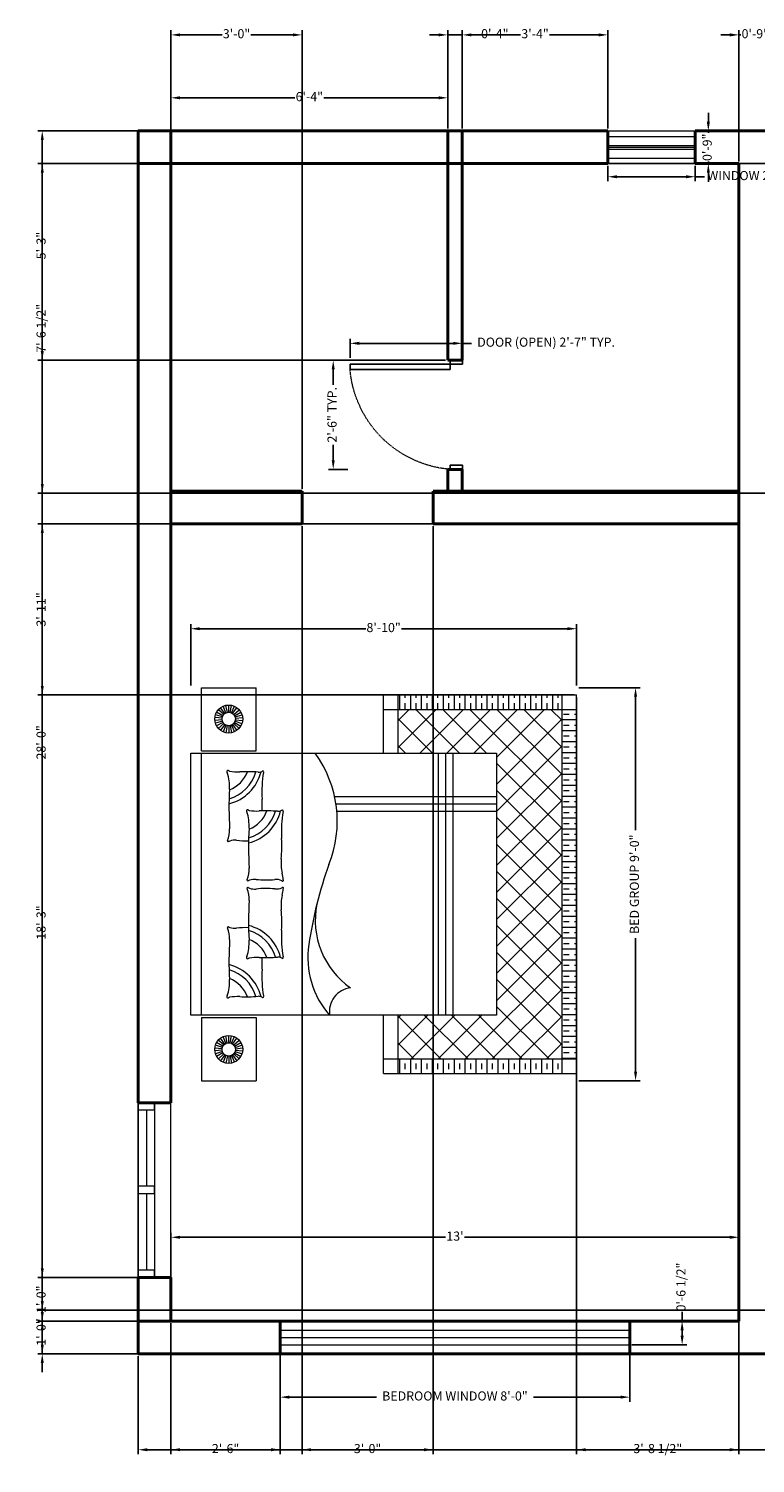
# Model space of a CAD drawing. Units: inches. Extents: x 3502 to 4078, y 3147 to 3541.
# Tile 1 of 3: x 3502 to 3702, y 3147 to 3541. Entities that reach past the tile are written whole.
import ezdxf

# ---------------------------------------------------------------- set-up
doc = ezdxf.new("R2010")
doc.units = ezdxf.units.IN
doc.linetypes.add('HIDDEN4', pattern=[0.09375, 0.0625, -0.03125])
doc.layers.get('0').update_dxf_attribs({"color": 255})
for name, color, linetype, lineweight in [('A-ANNO-DIMS', 2, 'Continuous', 18), ('A-FURN', 8, 'Continuous', 18), ('A-WALL', 7, 'Continuous', 40), ('A-WINDOW', 5, 'Continuous', 15)]:
    doc.layers.add(name, color=color, linetype=linetype, lineweight=lineweight)
doc.layers.add('A-DOOR', color=32, linetype='Continuous', lineweight=25, true_color=0xcd6928)
doc.layers.add('A-DOOR-SWNG', color=32, linetype='HIDDEN4', lineweight=13, true_color=0xcd6928)
doc.styles.get("Standard").update_dxf_attribs({"font": 'arial.ttf'})
doc.dimstyles.new('ISO-25', dxfattribs={"dimtxt": 2.5, "dimasz": 2.5, "dimexe": 1.25, "dimexo": 0.625, "dimtad": 0, "dimlunit": 4, "dimtxsty": 'Standard', "dimcen": 2.5, "dimadec": 0, "dimazin": 0, "dimtfac": 1, "dimtmove": 0, "dimatfit": 3, "dimfxl": 1, "dimarcsym": 0})

# ---------------------------------------------------------------- blocks, each defined once
blk = doc.blocks.new('*D2')
at = {"layer": 'A-ANNO-DIMS', "color": 0, "lineweight": -2, "transparency": 16777216}
for p, q in [((3541.21, 3513.35), (3541.21, 3523.06)), ((3543.71, 3521.81), (3575.25, 3521.81)), ((3614.71, 3521.81), (3583.16, 3521.81)), ((3617.21, 3513.35), (3617.21, 3523.06))]:
    blk.add_line(p, q, dxfattribs=at)
at = {"layer": 'A-ANNO-DIMS', "color": 0, "transparency": 16777216}
for points in [[(3543.71, 3522.23), (3543.71, 3521.39), (3541.21, 3521.81)], [(3614.71, 3522.23), (3614.71, 3521.39), (3617.21, 3521.81)]]:
    blk.add_solid(points, dxfattribs=at)
at = {"layer": 'Defpoints', "color": 0, "transparency": 16777216}
for p in [(3617.21, 3521.81), (3541.21, 3512.72), (3617.21, 3512.72)]:
    blk.add_point(p, dxfattribs=at)
at = {"layer": 'A-ANNO-DIMS', "color": 0, "transparency": 16777216, "insert": (3579.21, 3521.81), "char_height": 2.5, "attachment_point": 5}
blk.add_mtext('6\'-4"', dxfattribs=at)
blk = doc.blocks.new('A$C63CB6BFC')
at = {"layer": 'A-WALL', "ltscale": 75}
for p, q in [((0, 9), (0, 0)), ((48, 9), (48, 0))]:
    blk.add_line(p, q, dxfattribs=at)
at = {"layer": 'A-WINDOW'}
for p, q in [((48, 9), (0, 9)), ((0, 9), (48, 9)), ((1.99, 4.5), (1.99, 9)), ((23.04, 9), (23.04, 4.5)), ((25.02, 4.5), (25.02, 9)), ((46.01, 9), (46.01, 4.5)), ((48, 4.5), (0, 4.5)), ((0, 4.5), (1.99, 4.5)), ((23.04, 6.75), (1.99, 6.75)), ((23.04, 4.5), (25.02, 4.5)), ((46.01, 6.75), (25.02, 6.75)), ((46.01, 4.5), (48, 4.5)), ((0, 0), (48, 0))]:
    blk.add_line(p, q, dxfattribs=at)
blk = doc.blocks.new('*D9')
at = {"layer": 'A-ANNO-DIMS', "color": 0, "lineweight": -2, "transparency": 16777216}
for p, q in [((3541.21, 3186.35), (3541.21, 3209.99)), ((3543.71, 3208.74), (3616.58, 3208.74)), ((3694.71, 3208.74), (3621.84, 3208.74)), ((3697.21, 3186.35), (3697.21, 3209.99))]:
    blk.add_line(p, q, dxfattribs=at)
at = {"layer": 'A-ANNO-DIMS', "color": 0, "transparency": 16777216}
for points in [[(3543.71, 3209.16), (3543.71, 3208.33), (3541.21, 3208.74)], [(3694.71, 3209.16), (3694.71, 3208.33), (3697.21, 3208.74)]]:
    blk.add_solid(points, dxfattribs=at)
at = {"layer": 'Defpoints', "color": 0, "transparency": 16777216}
for p in [(3697.21, 3208.74), (3541.21, 3185.72), (3697.21, 3185.72)]:
    blk.add_point(p, dxfattribs=at)
at = {"layer": 'A-ANNO-DIMS', "color": 0, "transparency": 16777216, "insert": (3619.21, 3208.74), "char_height": 2.5, "attachment_point": 5}
blk.add_mtext("13'", dxfattribs=at)
blk = doc.blocks.new('BED')
h = blk.add_hatch()
h.set_pattern_fill('TRANS', color=256, scale=12, style=0)
h.set_pattern_definition([(360, (4433.967, -9715.0492), (1e-15, 3), []), (360, (4433.967, -9713.5492), (1e-15, 3), [1.5, -1.5])])
h.paths.add_polyline_path([(48, -103), (52, -103), (52, -58), (48, -58)])
h.paths.add_polyline_path([(-48, -58), (-52, -58), (-52, -103), (-48, -103)])
h = blk.add_hatch()
h.set_pattern_fill('ANSI37', color=256, scale=42, angle=-90, style=0)
h.set_pattern_definition([(315, (7787.1367, 4477.8466), (3.7123106, 3.7123106), []), (45, (7787.1367, 4477.8466), (-3.7123106, 3.7123106), [])])
h.paths.add_polyline_path([(-36, -85), (-36, -58), (-48, -58), (-48, -103), (48, -103), (48, -58), (36, -58), (36, -85)])
h = blk.add_hatch()
h.set_pattern_fill('TRANS', color=256, scale=12, angle=-90, style=0)
h.set_pattern_definition([(270, (4433.967, -9715.0492), (3, -1e-15), []), (270, (4435.467, -9715.0492), (3, -1e-15), [1.5, -1.5])])
h.paths.add_polyline_path([(48, -107), (48, -103), (-48, -103), (-48, -107)])
for p, q in [((-36, -1), (36, -1)), ((-36, -85), (-36, -1)), ((36, -1), (36, -85)), ((-54, -4), (-54, -19)), ((-36.64, -4), (-54, -4)), ((-45.96, -9.7), (-46.58, -7.8)), ((-45.58, -9.62), (-45.8, -7.63)), ((-45.2, -9.62), (-45, -7.63)), ((-44.82, -9.7), (-44.21, -7.79)), ((-36.64, -4), (-36.64, -19)), ((-36, -4), (36, -4)), ((36.64, -4), (36.64, -19)), ((36.64, -4), (54, -4)), ((44.82, -9.7), (44.21, -7.79)), ((45.2, -9.62), (45, -7.63)), ((45.58, -9.62), (45.8, -7.63)), ((45.96, -9.7), (46.58, -7.8)), ((54, -4), (54, -19)), ((-47.23, -11.45), (-49.23, -11.45)), ((-47.19, -11.07), (-49.14, -10.66)), ((-47.07, -10.7), (-48.9, -9.89)), ((-46.88, -10.37), (-48.5, -9.2)), ((-46.62, -10.08), (-47.96, -8.6)), ((-46.31, -9.86), (-47.31, -8.13)), ((-44.47, -9.85), (-43.48, -8.12)), ((-44.16, -10.08), (-42.83, -8.59)), ((-43.9, -10.36), (-42.29, -9.18)), ((-43.71, -10.7), (-41.89, -9.88)), ((-43.59, -11.06), (-41.64, -10.64)), ((-43.55, -11.44), (-41.55, -11.44)), ((43.55, -11.44), (41.55, -11.44)), ((43.59, -11.06), (41.64, -10.64)), ((43.71, -10.7), (41.89, -9.88)), ((43.9, -10.36), (42.29, -9.18)), ((44.16, -10.08), (42.83, -8.59)), ((44.47, -9.85), (43.48, -8.12)), ((46.31, -9.86), (47.31, -8.13)), ((46.62, -10.08), (47.96, -8.6)), ((46.88, -10.37), (48.5, -9.2)), ((47.07, -10.7), (48.9, -9.89)), ((47.19, -11.07), (49.14, -10.66)), ((47.23, -11.45), (49.23, -11.45)), ((-47.19, -11.83), (-49.14, -12.25)), ((-47.07, -12.2), (-48.89, -13.01)), ((-46.87, -12.53), (-48.49, -13.71)), ((-46.62, -12.81), (-47.95, -14.3)), ((-46.3, -13.04), (-47.3, -14.77)), ((-45.95, -13.2), (-46.57, -15.1)), ((-45.58, -13.27), (-45.78, -15.26)), ((-45.19, -13.27), (-44.98, -15.26)), ((-44.82, -13.19), (-44.2, -15.09)), ((-44.47, -13.04), (-43.46, -14.77)), ((-44.16, -12.81), (-42.82, -14.29)), ((-43.9, -12.52), (-42.28, -13.7)), ((-43.71, -12.19), (-41.88, -13)), ((-43.59, -11.83), (-41.63, -12.24)), ((43.59, -11.83), (41.63, -12.24)), ((43.71, -12.19), (41.88, -13)), ((43.9, -12.52), (42.28, -13.7)), ((44.16, -12.81), (42.82, -14.29)), ((44.47, -13.04), (43.46, -14.77)), ((44.82, -13.19), (44.2, -15.09)), ((45.19, -13.27), (44.98, -15.26)), ((45.58, -13.27), (45.78, -15.26)), ((45.95, -13.2), (46.57, -15.1)), ((46.3, -13.04), (47.3, -14.77)), ((46.62, -12.81), (47.95, -14.3)), ((46.87, -12.53), (48.49, -13.71)), ((47.07, -12.2), (48.89, -13.01)), ((47.19, -11.83), (49.14, -12.25)), ((-36.64, -19), (-54, -19)), ((36.64, -19), (54, -19)), ((20, -85), (20, -41.14)), ((22, -85), (22, -40.91)), ((24, -85), (24, -40.55)), ((-52, -54), (-52, -107)), ((-52, -54), (-36, -54)), ((-48, -54), (-48, -107)), ((36, -54), (52, -54)), ((48, -54), (48, -107)), ((52, -54), (52, -107)), ((-52, -58), (-36, -58)), ((36, -58), (52, -58)), ((36, -69), (-36, -69)), ((36, -71), (-36, -71)), ((36, -73), (-36, -73)), ((36, -85), (-36, -85)), ((-52, -103), (52, -103)), ((-52, -107), (52, -107))]:
    blk.add_line(p, q)
for centre, radius in [((-45.39, -11.45), 3.84), ((45.39, -11.45), 3.84), ((-45.39, -11.45), 1.84), ((45.39, -11.45), 1.84)]:
    blk.add_circle(centre, radius)
for centre, radius, start, end in [((-30.92, -11.24), 0.328, 35.8976, 208.6272), ((-42.38, -17.5), 12.73, 27.1629, 28.6272), ((-44.37, -13.89), 13.5, 357.4804, 9.3956), ((-33.8, -8.61), 8.46, 289.8695, 338.9843), ((-33.8, -8.61), 12.06, 283.8498, 346.0842), ((-33.8, -8.61), 10.71, 286.0319, 344.1205), ((-26.84, 0.13), 11.82, 251.1782, 273.3982), ((-20.92, -99.64), 88.13, 86.2964, 93.3982), ((-14.79, -4.98), 6.73, 266.2964, 294.303), ((-8.24, -13.16), 3.86, 159.0146, 186.273), ((-11.92, -11.33), 0.242, 335.7259, 114.303), ((-5.69, -14.14), 6.59, 155.7259, 159.0146), ((11.92, -11.33), 0.242, 65.697, 204.2741), ((5.69, -14.14), 6.59, 20.9854, 24.2741), ((8.24, -13.16), 3.86, 353.727, 20.9854), ((14.79, -4.98), 6.73, 245.697, 273.7036), ((20.92, -99.64), 88.13, 86.6018, 93.7036), ((33.8, -8.61), 12.06, 193.9158, 256.1502), ((33.8, -8.61), 10.71, 195.8795, 253.9681), ((33.8, -8.61), 8.46, 201.0157, 250.1305), ((26.84, 0.13), 11.82, 266.6018, 288.8218), ((30.92, -11.24), 0.328, 331.3728, 144.1024), ((44.37, -13.89), 13.5, 170.6044, 182.5196), ((42.38, -17.5), 12.73, 151.3728, 152.8371), ((10.15, -16.29), 41.07, 177.4804, 184.5075), ((-36.64, -16.28), 24.71, 358.5721, 6.273), ((36.64, -16.28), 24.71, 173.727, 181.4279), ((-10.15, -16.29), 41.07, 355.4925, 2.5196), ((-32.67, -19.67), 1.88, 339.2246, 4.5075), ((-20.16, -16.62), 0.328, 35.8976, 208.6272), ((-31.62, -22.87), 12.73, 27.1629, 28.6272), ((-33.61, -19.26), 13.5, 357.4804, 9.3956), ((-23.04, -13.99), 8.46, 289.8695, 338.9843), ((-23.04, -13.99), 12.06, 283.8498, 346.0842), ((-23.04, -13.99), 10.71, 286.0319, 344.1205), ((-16.08, -5.24), 11.82, 251.1782, 273.3982), ((-10.15, -105.01), 88.13, 86.2964, 93.3982), ((-4.03, -10.35), 6.73, 266.2964, 294.303), ((2.52, -18.53), 3.86, 159.0146, 186.273), ((-25.88, -21.66), 24.71, 354.3784, 6.273), ((-1.16, -16.7), 0.242, 335.7259, 114.303), ((5.07, -19.51), 6.59, 155.7259, 159.0146), ((1.16, -16.7), 0.242, 65.697, 204.2741), ((-5.07, -19.51), 6.59, 20.9854, 24.2741), ((-2.52, -18.53), 3.86, 353.727, 20.9854), ((25.88, -21.66), 24.71, 173.727, 185.6216), ((4.03, -10.35), 6.73, 245.697, 273.7036), ((10.15, -105.01), 88.13, 86.6018, 93.7036), ((23.04, -13.99), 12.06, 193.9158, 256.1502), ((23.04, -13.99), 10.71, 195.8795, 253.9681), ((23.04, -13.99), 8.46, 201.0157, 250.1305), ((16.08, -5.24), 11.82, 266.6018, 288.8218), ((20.16, -16.62), 0.328, 331.3728, 144.1024), ((33.61, -19.26), 13.5, 170.6044, 182.5196), ((31.62, -22.87), 12.73, 151.3728, 152.8371), ((32.67, -19.67), 1.88, 175.4925, 200.7754), ((-30.88, -20.82), 0.25, 147.6219, 311.9343), ((-32.72, -19.65), 1.93, 327.6219, 339.2246), ((-25.16, -53.53), 33, 93.5164, 99.6766), ((-25.27, -51.86), 31.33, 86.4836, 93.5164), ((-21.12, 15.68), 36.34, 266.4836, 271.5234), ((20.91, -21.66), 41.07, 177.4804, 184.5075), ((-20.91, -21.66), 41.07, 355.4925, 2.5196), ((21.12, 15.68), 36.34, 268.4766, 273.5164), ((25.27, -51.86), 31.33, 86.4836, 93.5164), ((25.16, -53.53), 33, 80.3234, 86.4836), ((30.88, -20.82), 0.25, 228.0657, 32.3781), ((32.72, -19.65), 1.93, 200.7754, 212.3781), ((-20.12, -26.19), 0.25, 147.6219, 311.9343), ((-21.96, -25.02), 1.93, 327.6219, 339.2246), ((-21.91, -25.04), 1.88, 339.2246, 4.5075), ((-14.4, -58.9), 33, 93.5164, 99.6766), ((-14.51, -57.23), 31.33, 86.4836, 93.5164), ((-10.35, 10.3), 36.34, 266.4836, 275.306), ((-5.78, -38.98), 13.15, 77.9645, 95.306), ((2.5, -0.17), 26.53, 257.9645, 261.9243), ((2.55, -24.46), 3.86, 174.3784, 204.7617), ((-1.09, -26.25), 0.228, 231.9005, 52.8902), ((1.09, -26.25), 0.228, 127.1098, 308.0995), ((-2.55, -24.46), 3.86, 335.2383, 5.6216), ((-2.5, -0.17), 26.53, 278.0757, 282.0355), ((5.78, -38.98), 13.15, 84.694, 102.0355), ((10.35, 10.3), 36.34, 264.694, 273.5164), ((14.51, -57.23), 31.33, 86.4836, 93.5164), ((14.4, -58.9), 33, 80.3234, 86.4836), ((20.12, -26.19), 0.25, 228.0657, 32.3781), ((21.91, -25.04), 1.88, 175.4925, 200.7754), ((21.96, -25.02), 1.93, 200.7754, 212.3781), ((-20.27, -56.85), 23.66, 81.0857, 131.6581), ((-9.91, -57.83), 22.61, 78.6456, 145.1521), ((-32.56, -143.87), 111.55, 70.0977, 81.7735), ((17.27, -9.21), 32.05, 248.2778, 305.7663), ((-34.97, -45.63), 6.55, 6.3172, 99.0807)]:
    blk.add_arc(centre, radius, start, end)
blk = doc.blocks.new('dfglkjdg')
at = {"layer": 'A-DOOR'}
for p, q in [((3245.28, 1353.69), (3245.28, 1357.7)), ((3245.28, 1357.7), (3246.64, 1357.7))]:
    blk.add_line(p, q, dxfattribs=at)
for points in [[(3210.73, 1357.7), (3212.09, 1357.7), (3212.09, 1353.69), (3210.73, 1353.69)], [(3210.73, 1353.69), (3210.73, 1357.7)], [(3245.28, 1353.69), (3246.64, 1353.69), (3246.64, 1357.7)]]:
    blk.add_lwpolyline(points, dxfattribs=at)
blk.add_lwpolyline([(3245.28, 1353.69), (3245.28, 1320.78), (3243.61, 1320.78), (3243.61, 1353.69)], close=True, dxfattribs=at)
at = {"layer": 'A-DOOR-SWNG'}
blk.add_arc((3246.64, 1356.69), 36.04, 184.7792, 265.1785, dxfattribs=at)
blk = doc.blocks.new('WIN-24IN')
for p, q in [((0, 7.5), (24, 7.5)), ((0, 5), (24, 5)), ((0, 4.5), (24, 4.5)), ((0, 4), (24, 4)), ((0, 1.5), (24, 1.5))]:
    blk.add_line(p, q)
blk.add_lwpolyline([(0, 9), (24, 9), (24, 0), (0, 0)], close=True)
blk = doc.blocks.new('WIN-96IN')
for p, q in [((0, 4), (96, 4)), ((50, 6.5), (50, 6.5)), ((0, 2), (96, 2)), ((0, 0), (96, 0))]:
    blk.add_line(p, q)
blk = doc.blocks.new('*D23')
at = {"layer": 'A-ANNO-DIMS', "color": 0, "lineweight": -2, "transparency": 16777216}
for p, q in [((3661.21, 3503.1), (3661.21, 3498.87)), ((3685.21, 3503.1), (3685.21, 3498.87)), ((3663.71, 3500.12), (3682.71, 3500.12)), ((3685.21, 3500.12), (3687.71, 3500.12))]:
    blk.add_line(p, q, dxfattribs=at)
at = {"layer": 'A-ANNO-DIMS', "color": 0, "transparency": 16777216}
for points in [[(3663.71, 3500.54), (3663.71, 3499.71), (3661.21, 3500.12)], [(3682.71, 3500.54), (3682.71, 3499.71), (3685.21, 3500.12)]]:
    blk.add_solid(points, dxfattribs=at)
at = {"layer": 'Defpoints', "color": 0, "transparency": 16777216}
for p in [(3661.21, 3503.72), (3685.21, 3503.72), (3685.21, 3500.12)]:
    blk.add_point(p, dxfattribs=at)
at = {"layer": 'A-ANNO-DIMS', "color": 0, "transparency": 16777216, "insert": (3699.86, 3500.12), "char_height": 2.5, "attachment_point": 5}
blk.add_mtext('WINDOW 2\'-0"', dxfattribs=at)
blk = doc.blocks.new('*D24')
at = {"layer": 'A-ANNO-DIMS', "color": 0, "lineweight": -2, "transparency": 16777216}
for p, q in [((3688.81, 3515.22), (3688.81, 3517.72)), ((3685.83, 3512.72), (3690.06, 3512.72)), ((3688.81, 3512.72), (3688.81, 3512.17)), ((3688.81, 3503.72), (3688.81, 3504.28)), ((3685.83, 3503.72), (3690.06, 3503.72)), ((3688.81, 3501.22), (3688.81, 3498.72))]:
    blk.add_line(p, q, dxfattribs=at)
at = {"layer": 'A-ANNO-DIMS', "color": 0, "transparency": 16777216}
for points in [[(3688.39, 3515.22), (3689.23, 3515.22), (3688.81, 3512.72)], [(3688.39, 3501.22), (3689.23, 3501.22), (3688.81, 3503.72)]]:
    blk.add_solid(points, dxfattribs=at)
at = {"layer": 'Defpoints', "color": 0, "transparency": 16777216}
for p in [(3685.21, 3512.72), (3688.81, 3512.72), (3685.21, 3503.72)]:
    blk.add_point(p, dxfattribs=at)
at = {"layer": 'A-ANNO-DIMS', "color": 0, "transparency": 16777216, "insert": (3688.81, 3508.22), "char_height": 2.5, "attachment_point": 5, "rotation": 90}
blk.add_mtext('0\'-9"', dxfattribs=at)
blk = doc.blocks.new('*D25')
at = {"layer": 'A-ANNO-DIMS', "color": 0, "lineweight": -2, "transparency": 16777216}
for p, q in [((3571.21, 3178.6), (3571.21, 3163.57)), ((3667.21, 3178.6), (3667.21, 3163.57)), ((3573.71, 3164.82), (3597.66, 3164.82)), ((3664.71, 3164.82), (3640.76, 3164.82))]:
    blk.add_line(p, q, dxfattribs=at)
at = {"layer": 'A-ANNO-DIMS', "color": 0, "transparency": 16777216}
for points in [[(3573.71, 3165.24), (3573.71, 3164.41), (3571.21, 3164.82)], [(3664.71, 3165.24), (3664.71, 3164.41), (3667.21, 3164.82)]]:
    blk.add_solid(points, dxfattribs=at)
at = {"layer": 'Defpoints', "color": 0, "transparency": 16777216}
for p in [(3571.21, 3179.22), (3667.21, 3179.22), (3667.21, 3164.82)]:
    blk.add_point(p, dxfattribs=at)
at = {"layer": 'A-ANNO-DIMS', "color": 0, "transparency": 16777216, "insert": (3619.21, 3164.82), "char_height": 2.5, "attachment_point": 5}
blk.add_mtext('BEDROOM WINDOW 8\'-0"', dxfattribs=at)
blk = doc.blocks.new('*D26')
at = {"layer": 'A-ANNO-DIMS', "color": 0, "lineweight": -2, "transparency": 16777216}
for p, q in [((3667.83, 3185.72), (3682.86, 3185.72)), ((3681.61, 3185.72), (3681.61, 3188.22)), ((3681.61, 3181.72), (3681.61, 3183.22)), ((3667.83, 3179.22), (3682.86, 3179.22))]:
    blk.add_line(p, q, dxfattribs=at)
at = {"layer": 'A-ANNO-DIMS', "color": 0, "transparency": 16777216}
for points in [[(3681.19, 3183.22), (3682.03, 3183.22), (3681.61, 3185.72)], [(3681.19, 3181.72), (3682.03, 3181.72), (3681.61, 3179.22)]]:
    blk.add_solid(points, dxfattribs=at)
at = {"layer": 'Defpoints', "color": 0, "transparency": 16777216}
for p in [(3667.21, 3185.72), (3681.61, 3185.72), (3667.21, 3179.22)]:
    blk.add_point(p, dxfattribs=at)
at = {"layer": 'A-ANNO-DIMS', "color": 0, "transparency": 16777216, "insert": (3681.61, 3195.08), "char_height": 2.5, "attachment_point": 5, "rotation": 90}
blk.add_mtext('0\'-6 1/2"', dxfattribs=at)
blk = doc.blocks.new('*D27')
at = {"layer": 'A-ANNO-DIMS', "color": 0, "lineweight": -2, "transparency": 16777216}
for p, q in [((3590.4, 3450.35), (3590.4, 3455.6)), ((3592.9, 3454.35), (3618.74, 3454.35)), ((3621.24, 3450.35), (3621.24, 3455.6)), ((3621.24, 3454.35), (3623.74, 3454.35))]:
    blk.add_line(p, q, dxfattribs=at)
at = {"layer": 'A-ANNO-DIMS', "color": 0, "transparency": 16777216}
for points in [[(3592.9, 3454.77), (3592.9, 3453.93), (3590.4, 3454.35)], [(3618.74, 3454.77), (3618.74, 3453.93), (3621.24, 3454.35)]]:
    blk.add_solid(points, dxfattribs=at)
at = {"layer": 'Defpoints', "color": 0, "transparency": 16777216}
for p in [(3621.24, 3454.35), (3590.4, 3449.72), (3621.24, 3449.72)]:
    blk.add_point(p, dxfattribs=at)
at = {"layer": 'A-ANNO-DIMS', "color": 0, "transparency": 16777216, "insert": (3644.24, 3454.35), "char_height": 2.5, "attachment_point": 5}
blk.add_mtext('DOOR (OPEN) 2\'-7" TYP.', dxfattribs=at)
blk = doc.blocks.new('*D28')
at = {"layer": 'A-ANNO-DIMS', "color": 0, "lineweight": -2, "transparency": 16777216}
for p, q in [((3589.78, 3449.72), (3584.52, 3449.72)), ((3585.77, 3447.22), (3585.77, 3442.99)), ((3585.77, 3422.22), (3585.77, 3426.46)), ((3589.78, 3419.72), (3584.52, 3419.72))]:
    blk.add_line(p, q, dxfattribs=at)
at = {"layer": 'A-ANNO-DIMS', "color": 0, "transparency": 16777216}
for points in [[(3585.36, 3447.22), (3586.19, 3447.22), (3585.77, 3449.72)], [(3585.36, 3422.22), (3586.19, 3422.22), (3585.77, 3419.72)]]:
    blk.add_solid(points, dxfattribs=at)
at = {"layer": 'Defpoints', "color": 0, "transparency": 16777216}
for p in [(3585.77, 3449.72), (3590.4, 3449.72), (3590.4, 3419.72)]:
    blk.add_point(p, dxfattribs=at)
at = {"layer": 'A-ANNO-DIMS', "color": 0, "transparency": 16777216, "insert": (3585.77, 3434.72), "char_height": 2.5, "attachment_point": 5, "rotation": 90}
blk.add_mtext('2\'-6" TYP.', dxfattribs=at)
blk = doc.blocks.new('*D29')
at = {"layer": 'A-ANNO-DIMS', "color": 0, "lineweight": -2, "transparency": 16777216}
for p, q in [((3653.25, 3359.74), (3670.07, 3359.74)), ((3668.82, 3357.24), (3668.82, 3320.6)), ((3668.82, 3254.24), (3668.82, 3290.88)), ((3653.25, 3251.74), (3670.07, 3251.74))]:
    blk.add_line(p, q, dxfattribs=at)
at = {"layer": 'A-ANNO-DIMS', "color": 0, "transparency": 16777216}
for points in [[(3668.4, 3357.24), (3669.24, 3357.24), (3668.82, 3359.74)], [(3668.4, 3254.24), (3669.24, 3254.24), (3668.82, 3251.74)]]:
    blk.add_solid(points, dxfattribs=at)
at = {"layer": 'Defpoints', "color": 0, "transparency": 16777216}
for p in [(3652.62, 3359.74), (3668.82, 3359.74), (3652.62, 3251.74)]:
    blk.add_point(p, dxfattribs=at)
at = {"layer": 'A-ANNO-DIMS', "color": 0, "transparency": 16777216, "insert": (3668.82, 3305.74), "char_height": 2.5, "attachment_point": 5, "rotation": 90}
blk.add_mtext('BED GROUP 9\'-0"', dxfattribs=at)
blk = doc.blocks.new('*D30')
at = {"layer": 'A-ANNO-DIMS', "color": 0, "lineweight": -2, "transparency": 16777216}
for p, q in [((3546.62, 3360.37), (3546.62, 3377.19)), ((3549.12, 3375.94), (3594.7, 3375.94)), ((3650.12, 3375.94), (3604.54, 3375.94)), ((3652.62, 3360.37), (3652.62, 3377.19))]:
    blk.add_line(p, q, dxfattribs=at)
at = {"layer": 'A-ANNO-DIMS', "color": 0, "transparency": 16777216}
for points in [[(3549.12, 3376.36), (3549.12, 3375.53), (3546.62, 3375.94)], [(3650.12, 3376.36), (3650.12, 3375.53), (3652.62, 3375.94)]]:
    blk.add_solid(points, dxfattribs=at)
at = {"layer": 'Defpoints', "color": 0, "transparency": 16777216}
for p in [(3546.62, 3375.94), (3546.62, 3359.74), (3652.62, 3359.74)]:
    blk.add_point(p, dxfattribs=at)
at = {"layer": 'A-ANNO-DIMS', "color": 0, "transparency": 16777216, "insert": (3599.62, 3375.94), "char_height": 2.5, "attachment_point": 5}
blk.add_mtext('8\'-10"', dxfattribs=at)
blk = doc.blocks.new('*D35')
at = {"layer": 'A-ANNO-DIMS', "color": 0, "lineweight": -2, "transparency": 16777216}
for p, q in [((3697.21, 3504.35), (3697.21, 3540.35)), ((3706.21, 3504.35), (3706.21, 3540.35)), ((3694.71, 3539.1), (3692.21, 3539.1)), ((3697.21, 3539.1), (3697.76, 3539.1)), ((3706.21, 3539.1), (3705.66, 3539.1)), ((3708.71, 3539.1), (3711.21, 3539.1))]:
    blk.add_line(p, q, dxfattribs=at)
at = {"layer": 'A-ANNO-DIMS', "color": 0, "transparency": 16777216}
for points in [[(3694.71, 3539.51), (3694.71, 3538.68), (3697.21, 3539.1)], [(3708.71, 3539.51), (3708.71, 3538.68), (3706.21, 3539.1)]]:
    blk.add_solid(points, dxfattribs=at)
at = {"layer": 'Defpoints', "color": 0, "transparency": 16777216}
for p in [(3706.21, 3539.1), (3697.21, 3503.72), (3706.21, 3503.72)]:
    blk.add_point(p, dxfattribs=at)
at = {"layer": 'A-ANNO-DIMS', "color": 0, "transparency": 16777216, "insert": (3701.71, 3539.1), "char_height": 2.5, "attachment_point": 5}
blk.add_mtext('0\'-9"', dxfattribs=at)
blk = doc.blocks.new('*D36')
at = {"layer": 'A-ANNO-DIMS', "color": 0, "lineweight": -2, "transparency": 16777216}
for p, q in [((3617.21, 3513.35), (3617.21, 3540.35)), ((3621.21, 3513.34), (3621.21, 3540.35)), ((3614.71, 3539.1), (3612.21, 3539.1)), ((3617.21, 3539.1), (3621.21, 3539.1)), ((3623.71, 3539.1), (3626.21, 3539.1))]:
    blk.add_line(p, q, dxfattribs=at)
at = {"layer": 'A-ANNO-DIMS', "color": 0, "transparency": 16777216}
for points in [[(3614.71, 3539.51), (3614.71, 3538.68), (3617.21, 3539.1)], [(3623.71, 3539.51), (3623.71, 3538.68), (3621.21, 3539.1)]]:
    blk.add_solid(points, dxfattribs=at)
at = {"layer": 'Defpoints', "color": 0, "transparency": 16777216}
for p in [(3621.21, 3539.1), (3617.21, 3512.72), (3621.21, 3512.72)]:
    blk.add_point(p, dxfattribs=at)
at = {"layer": 'A-ANNO-DIMS', "color": 0, "transparency": 16777216, "insert": (3630.16, 3539.1), "char_height": 2.5, "attachment_point": 5}
blk.add_mtext('0\'-4"', dxfattribs=at)
blk = doc.blocks.new('*D38')
at = {"layer": 'A-ANNO-DIMS', "color": 0, "lineweight": -2, "transparency": 16777216}
for p, q in [((3621.21, 3513.34), (3621.21, 3540.35)), ((3661.21, 3513.35), (3661.21, 3540.35)), ((3623.71, 3539.1), (3637.26, 3539.1)), ((3658.71, 3539.1), (3645.16, 3539.1))]:
    blk.add_line(p, q, dxfattribs=at)
at = {"layer": 'A-ANNO-DIMS', "color": 0, "transparency": 16777216}
for points in [[(3623.71, 3539.51), (3623.71, 3538.68), (3621.21, 3539.1)], [(3658.71, 3539.51), (3658.71, 3538.68), (3661.21, 3539.1)]]:
    blk.add_solid(points, dxfattribs=at)
at = {"layer": 'Defpoints', "color": 0, "transparency": 16777216}
for p in [(3661.21, 3539.1), (3621.21, 3512.72), (3661.21, 3512.72)]:
    blk.add_point(p, dxfattribs=at)
at = {"layer": 'A-ANNO-DIMS', "color": 0, "transparency": 16777216, "insert": (3641.21, 3539.1), "char_height": 2.5, "attachment_point": 5}
blk.add_mtext('3\'-4"', dxfattribs=at)
blk = doc.blocks.new('*D41')
at = {"layer": 'A-ANNO-DIMS', "color": 0, "lineweight": -2, "transparency": 16777216}
for p, q in [((3696.58, 3404.72), (3504.6, 3404.72)), ((3505.85, 3402.22), (3505.85, 3300.02)), ((3505.85, 3188.22), (3505.85, 3290.42)), ((3696.58, 3185.72), (3504.6, 3185.72))]:
    blk.add_line(p, q, dxfattribs=at)
at = {"layer": 'A-ANNO-DIMS', "color": 0, "transparency": 16777216}
for points in [[(3505.44, 3402.22), (3506.27, 3402.22), (3505.85, 3404.72)], [(3505.44, 3188.22), (3506.27, 3188.22), (3505.85, 3185.72)]]:
    blk.add_solid(points, dxfattribs=at)
at = {"layer": 'Defpoints', "color": 0, "transparency": 16777216}
for p in [(3505.85, 3404.72), (3697.21, 3404.72), (3697.21, 3185.72)]:
    blk.add_point(p, dxfattribs=at)
at = {"layer": 'A-ANNO-DIMS', "color": 0, "transparency": 16777216, "insert": (3505.85, 3295.22), "char_height": 2.5, "attachment_point": 5, "rotation": 90}
blk.add_mtext('18\'-3"', dxfattribs=at)
blk = doc.blocks.new('*D47')
at = {"layer": 'A-ANNO-DIMS', "color": 0, "lineweight": -2, "transparency": 16777216}
for p, q in [((3541.21, 3185.1), (3541.21, 3149.12)), ((3571.21, 3185.1), (3571.21, 3149.12)), ((3543.71, 3150.37), (3552.24, 3150.37)), ((3568.71, 3150.37), (3560.18, 3150.37))]:
    blk.add_line(p, q, dxfattribs=at)
at = {"layer": 'A-ANNO-DIMS', "color": 0, "transparency": 16777216}
for points in [[(3543.71, 3150.79), (3543.71, 3149.95), (3541.21, 3150.37)], [(3568.71, 3150.79), (3568.71, 3149.95), (3571.21, 3150.37)]]:
    blk.add_solid(points, dxfattribs=at)
at = {"layer": 'Defpoints', "color": 0, "transparency": 16777216}
for p in [(3541.21, 3185.72), (3571.21, 3185.72), (3571.21, 3150.37)]:
    blk.add_point(p, dxfattribs=at)
at = {"layer": 'A-ANNO-DIMS', "color": 0, "transparency": 16777216, "insert": (3556.21, 3150.37), "char_height": 2.5, "attachment_point": 5}
blk.add_mtext('2\'-6"', dxfattribs=at)
blk = doc.blocks.new('*D48')
at = {"layer": 'A-ANNO-DIMS', "color": 0, "lineweight": -2, "transparency": 16777216}
for p, q in [((3505.85, 3191.22), (3505.85, 3193.72)), ((3705.58, 3188.72), (3504.6, 3188.72)), ((3505.85, 3188.72), (3505.85, 3186.55)), ((3505.85, 3176.72), (3505.85, 3178.89)), ((3705.58, 3176.72), (3504.6, 3176.72)), ((3505.85, 3174.22), (3505.85, 3171.72))]:
    blk.add_line(p, q, dxfattribs=at)
at = {"layer": 'A-ANNO-DIMS', "color": 0, "transparency": 16777216}
for points in [[(3505.44, 3191.22), (3506.27, 3191.22), (3505.85, 3188.72)], [(3505.44, 3174.22), (3506.27, 3174.22), (3505.85, 3176.72)]]:
    blk.add_solid(points, dxfattribs=at)
at = {"layer": 'Defpoints', "color": 0, "transparency": 16777216}
for p in [(3505.85, 3188.72), (3706.21, 3188.72), (3706.21, 3176.72)]:
    blk.add_point(p, dxfattribs=at)
at = {"layer": 'A-ANNO-DIMS', "color": 0, "transparency": 16777216, "insert": (3505.85, 3182.72), "char_height": 2.5, "attachment_point": 5, "rotation": 90}
blk.add_mtext('1\'-0"', dxfattribs=at)
blk = doc.blocks.new('*D49')
at = {"layer": 'A-ANNO-DIMS', "color": 0, "lineweight": -2, "transparency": 16777216}
for p, q in [((3577.21, 3404.1), (3577.21, 3149.12)), ((3613.21, 3404.1), (3613.21, 3149.12)), ((3579.71, 3150.37), (3591.26, 3150.37)), ((3610.71, 3150.37), (3599.16, 3150.37))]:
    blk.add_line(p, q, dxfattribs=at)
at = {"layer": 'A-ANNO-DIMS', "color": 0, "transparency": 16777216}
for points in [[(3579.71, 3150.79), (3579.71, 3149.95), (3577.21, 3150.37)], [(3610.71, 3150.79), (3610.71, 3149.95), (3613.21, 3150.37)]]:
    blk.add_solid(points, dxfattribs=at)
at = {"layer": 'Defpoints', "color": 0, "transparency": 16777216}
for p in [(3577.21, 3404.72), (3613.21, 3404.72), (3613.21, 3150.37)]:
    blk.add_point(p, dxfattribs=at)
at = {"layer": 'A-ANNO-DIMS', "color": 0, "transparency": 16777216, "insert": (3595.21, 3150.37), "char_height": 2.5, "attachment_point": 5}
blk.add_mtext('3\'-0"', dxfattribs=at)
blk = doc.blocks.new('*D50')
at = {"layer": 'A-ANNO-DIMS', "color": 0, "lineweight": -2, "transparency": 16777216}
for p, q in [((3541.21, 3414.35), (3541.21, 3540.35)), ((3577.21, 3414.35), (3577.21, 3540.35)), ((3543.71, 3539.1), (3555.26, 3539.1)), ((3574.71, 3539.1), (3563.16, 3539.1))]:
    blk.add_line(p, q, dxfattribs=at)
at = {"layer": 'A-ANNO-DIMS', "color": 0, "transparency": 16777216}
for points in [[(3543.71, 3539.51), (3543.71, 3538.68), (3541.21, 3539.1)], [(3574.71, 3539.51), (3574.71, 3538.68), (3577.21, 3539.1)]]:
    blk.add_solid(points, dxfattribs=at)
at = {"layer": 'Defpoints', "color": 0, "transparency": 16777216}
for p in [(3577.21, 3539.1), (3541.21, 3413.72), (3577.21, 3413.72)]:
    blk.add_point(p, dxfattribs=at)
at = {"layer": 'A-ANNO-DIMS', "color": 0, "transparency": 16777216, "insert": (3559.21, 3539.1), "char_height": 2.5, "attachment_point": 5}
blk.add_mtext('3\'-0"', dxfattribs=at)
blk = doc.blocks.new('*D51')
at = {"layer": 'A-ANNO-DIMS', "color": 0, "lineweight": -2, "transparency": 16777216}
for p, q in [((3616.58, 3512.72), (3504.6, 3512.72)), ((3505.85, 3510.22), (3505.85, 3485.17)), ((3505.85, 3452.22), (3505.85, 3477.28)), ((3616.58, 3449.72), (3504.6, 3449.72))]:
    blk.add_line(p, q, dxfattribs=at)
at = {"layer": 'A-ANNO-DIMS', "color": 0, "transparency": 16777216}
for points in [[(3505.44, 3510.22), (3506.27, 3510.22), (3505.85, 3512.72)], [(3505.44, 3452.22), (3506.27, 3452.22), (3505.85, 3449.72)]]:
    blk.add_solid(points, dxfattribs=at)
at = {"layer": 'Defpoints', "color": 0, "transparency": 16777216}
for p in [(3617.21, 3512.72), (3505.85, 3449.72), (3617.21, 3449.72)]:
    blk.add_point(p, dxfattribs=at)
at = {"layer": 'A-ANNO-DIMS', "color": 0, "transparency": 16777216, "insert": (3505.85, 3481.22), "char_height": 2.5, "attachment_point": 5, "rotation": 90}
blk.add_mtext('5\'-3"', dxfattribs=at)
blk = doc.blocks.new('*D53')
at = {"layer": 'A-ANNO-DIMS', "color": 0, "lineweight": -2, "transparency": 16777216}
for p, q in [((3505.85, 3200.22), (3505.85, 3202.72)), ((3540.58, 3197.72), (3504.6, 3197.72)), ((3505.85, 3197.72), (3505.85, 3195.55)), ((3540.58, 3185.72), (3504.6, 3185.72)), ((3505.85, 3185.72), (3505.85, 3187.89)), ((3505.85, 3183.22), (3505.85, 3180.72))]:
    blk.add_line(p, q, dxfattribs=at)
at = {"layer": 'A-ANNO-DIMS', "color": 0, "transparency": 16777216}
for points in [[(3505.44, 3200.22), (3506.27, 3200.22), (3505.85, 3197.72)], [(3505.44, 3183.22), (3506.27, 3183.22), (3505.85, 3185.72)]]:
    blk.add_solid(points, dxfattribs=at)
at = {"layer": 'Defpoints', "color": 0, "transparency": 16777216}
for p in [(3505.85, 3197.72), (3541.21, 3197.72), (3541.21, 3185.72)]:
    blk.add_point(p, dxfattribs=at)
at = {"layer": 'A-ANNO-DIMS', "color": 0, "transparency": 16777216, "insert": (3505.85, 3191.72), "char_height": 2.5, "attachment_point": 5, "rotation": 90}
blk.add_mtext('1\'-0"', dxfattribs=at)
blk = doc.blocks.new('*D55')
at = {"layer": 'A-ANNO-DIMS', "color": 0, "lineweight": -2, "transparency": 16777216}
for p, q in [((4038.58, 3503.72), (3504.6, 3503.72)), ((3505.85, 3501.22), (3505.85, 3465.32)), ((3505.85, 3415.71), (3505.85, 3451.62)), ((4038.58, 3413.21), (3504.6, 3413.21))]:
    blk.add_line(p, q, dxfattribs=at)
at = {"layer": 'A-ANNO-DIMS', "color": 0, "transparency": 16777216}
for points in [[(3505.44, 3501.22), (3506.27, 3501.22), (3505.85, 3503.72)], [(3505.44, 3415.71), (3506.27, 3415.71), (3505.85, 3413.21)]]:
    blk.add_solid(points, dxfattribs=at)
at = {"layer": 'Defpoints', "color": 0, "transparency": 16777216}
for p in [(3505.85, 3503.72), (4039.21, 3503.72), (4039.21, 3413.21)]:
    blk.add_point(p, dxfattribs=at)
at = {"layer": 'A-ANNO-DIMS', "color": 0, "transparency": 16777216, "insert": (3505.85, 3458.47), "char_height": 2.5, "attachment_point": 5, "rotation": 90}
blk.add_mtext('7\'-6 1/2"', dxfattribs=at)
blk = doc.blocks.new('*D56')
at = {"layer": 'A-ANNO-DIMS', "color": 0, "lineweight": -2, "transparency": 16777216}
for p, q in [((3531.58, 3512.72), (3504.6, 3512.72)), ((3505.85, 3510.22), (3505.85, 3349.66)), ((3505.85, 3179.22), (3505.85, 3339.78)), ((3531.58, 3176.72), (3504.6, 3176.72))]:
    blk.add_line(p, q, dxfattribs=at)
at = {"layer": 'A-ANNO-DIMS', "color": 0, "transparency": 16777216}
for points in [[(3505.44, 3510.22), (3506.27, 3510.22), (3505.85, 3512.72)], [(3505.44, 3179.22), (3506.27, 3179.22), (3505.85, 3176.72)]]:
    blk.add_solid(points, dxfattribs=at)
at = {"layer": 'Defpoints', "color": 0, "transparency": 16777216}
for p in [(3505.85, 3512.72), (3532.21, 3512.72), (3532.21, 3176.72)]:
    blk.add_point(p, dxfattribs=at)
at = {"layer": 'A-ANNO-DIMS', "color": 0, "transparency": 16777216, "insert": (3505.85, 3344.72), "char_height": 2.5, "attachment_point": 5, "rotation": 90}
blk.add_mtext('28\'-0"', dxfattribs=at)
blk = doc.blocks.new('*D57')
at = {"layer": 'A-ANNO-DIMS', "color": 0, "lineweight": -2, "transparency": 16777216}
for p, q in [((3532.21, 3176.1), (3532.21, 3149.12)), ((4048.21, 3176.1), (4048.21, 3149.12)), ((3534.71, 3150.37), (3785.24, 3150.37)), ((4045.71, 3150.37), (3795.18, 3150.37))]:
    blk.add_line(p, q, dxfattribs=at)
at = {"layer": 'A-ANNO-DIMS', "color": 0, "transparency": 16777216}
for points in [[(3534.71, 3150.79), (3534.71, 3149.95), (3532.21, 3150.37)], [(4045.71, 3150.79), (4045.71, 3149.95), (4048.21, 3150.37)]]:
    blk.add_solid(points, dxfattribs=at)
at = {"layer": 'Defpoints', "color": 0, "transparency": 16777216}
for p in [(3532.21, 3176.72), (4048.21, 3176.72), (4048.21, 3150.37)]:
    blk.add_point(p, dxfattribs=at)
at = {"layer": 'A-ANNO-DIMS', "color": 0, "transparency": 16777216, "insert": (3790.21, 3150.37), "char_height": 2.5, "attachment_point": 5}
blk.add_mtext('43\'-0"', dxfattribs=at)
blk = doc.blocks.new('*D58')
at = {"layer": 'A-ANNO-DIMS', "color": 0, "lineweight": -2, "transparency": 16777216}
for p, q in [((3697.21, 3404.1), (3697.21, 3149.12)), ((3652.62, 3357.12), (3652.62, 3149.12)), ((3655.12, 3150.37), (3668.06, 3150.37)), ((3694.71, 3150.37), (3681.77, 3150.37))]:
    blk.add_line(p, q, dxfattribs=at)
at = {"layer": 'A-ANNO-DIMS', "color": 0, "transparency": 16777216}
for points in [[(3655.12, 3150.79), (3655.12, 3149.95), (3652.62, 3150.37)], [(3694.71, 3150.79), (3694.71, 3149.95), (3697.21, 3150.37)]]:
    blk.add_solid(points, dxfattribs=at)
at = {"layer": 'Defpoints', "color": 0, "transparency": 16777216}
for p in [(3697.21, 3404.72), (3652.62, 3357.74), (3697.21, 3150.37)]:
    blk.add_point(p, dxfattribs=at)
at = {"layer": 'A-ANNO-DIMS', "color": 0, "transparency": 16777216, "insert": (3674.92, 3150.37), "char_height": 2.5, "attachment_point": 5}
blk.add_mtext('3\'-8 1/2"', dxfattribs=at)
blk = doc.blocks.new('*D59')
at = {"layer": 'A-ANNO-DIMS', "color": 0, "lineweight": -2, "transparency": 16777216}
for p, q in [((3696.58, 3404.72), (3504.6, 3404.72)), ((3505.85, 3402.22), (3505.85, 3386.15)), ((3505.85, 3360.24), (3505.85, 3376.31)), ((3652, 3357.74), (3504.6, 3357.74))]:
    blk.add_line(p, q, dxfattribs=at)
at = {"layer": 'A-ANNO-DIMS', "color": 0, "transparency": 16777216}
for points in [[(3505.44, 3402.22), (3506.27, 3402.22), (3505.85, 3404.72)], [(3505.44, 3360.24), (3506.27, 3360.24), (3505.85, 3357.74)]]:
    blk.add_solid(points, dxfattribs=at)
at = {"layer": 'Defpoints', "color": 0, "transparency": 16777216}
for p in [(3505.85, 3404.72), (3697.21, 3404.72), (3652.62, 3357.74)]:
    blk.add_point(p, dxfattribs=at)
at = {"layer": 'A-ANNO-DIMS', "color": 0, "transparency": 16777216, "insert": (3505.85, 3381.23), "char_height": 2.5, "attachment_point": 5, "rotation": 90}
blk.add_mtext('3\'-11"', dxfattribs=at)

msp = doc.modelspace()

# ---------------------------------------------------------------- linework, layer by layer
at = {"layer": 'A-WALL'}
for p, q in [((3541.21, 3503.724), (3541.21, 3512.724)), ((3617.21, 3449.724), (3617.21, 3512.724)), ((3621.21, 3449.724), (3621.21, 3512.72)), ((3661.21, 3503.724), (3661.21, 3512.724)), ((3685.21, 3503.724), (3685.21, 3512.724)), ((3541.21, 3503.724), (3532.21, 3503.724)), ((3697.21, 3185.72), (3697.21, 3503.724)), ((3617.21, 3449.724), (3621.21, 3449.724)), ((3617.21, 3413.724), (3617.21, 3419.724)), ((3617.21, 3419.724), (3621.21, 3419.724)), ((3621.21, 3413.724), (3621.21, 3419.724)), ((3541.21, 3404.724), (3541.21, 3413.724)), ((3577.21, 3413.724), (3541.21, 3413.724)), ((3577.21, 3404.724), (3577.21, 3413.724)), ((3617.21, 3413.724), (3613.21, 3413.724)), ((3613.21, 3404.724), (3613.21, 3413.724)), ((3617.21, 3413.724), (3621.21, 3413.724)), ((3697.21, 3413.724), (3621.21, 3413.724)), ((3577.21, 3404.724), (3541.21, 3404.724)), ((3697.21, 3404.724), (3613.21, 3404.724)), ((3541.21, 3245.724), (3532.21, 3245.724)), ((3541.21, 3197.724), (3532.21, 3197.724)), ((3541.21, 3185.724), (3532.21, 3185.724)), ((3571.21, 3185.724), (3571.21, 3176.724)), ((3667.21, 3185.724), (3667.21, 3176.724))]:
    msp.add_line(p, q, dxfattribs=at)
for points in [[(3532.21, 3245.724), (3532.21, 3512.724), (3661.21, 3512.724)], [(3685.21, 3512.724), (3907.21, 3512.724)], [(3541.21, 3413.724), (3541.21, 3503.724), (3661.21, 3503.724)], [(3685.21, 3503.724), (3697.21, 3503.724)], [(3541.21, 3245.724), (3541.21, 3404.724)], [(3706.21, 3176.724), (3532.21, 3176.724), (3532.21, 3197.724)], [(3697.21, 3185.724), (3541.21, 3185.724), (3541.21, 3197.724)]]:
    msp.add_lwpolyline(points, dxfattribs=at)

# ---------------------------------------------------------------- block references
at = {"layer": 'A-DOOR', "xscale": -0.8352314093545642, "yscale": 0.8352314093545642, "zscale": 0.8352314093545642, "rotation": 270}
msp.add_blockref('dfglkjdg', (2487.247, 738.025), dxfattribs=at)
at = {"layer": 'A-FURN', "rotation": 90}
msp.add_blockref('BED', (3545.621, 3305.742), dxfattribs=at)
at = {"layer": 'A-WINDOW'}
for name, p in [('WIN-24IN', (3661.21, 3503.724)), ('WIN-96IN', (3571.21, 3179.224))]:
    msp.add_blockref(name, p, dxfattribs=at)
at = {"layer": 'A-WINDOW', "rotation": 90}
msp.add_blockref('A$C63CB6BFC', (3541.21, 3197.724), dxfattribs=at)

# ---------------------------------------------------------------- dimensions: what is measured, and where the dimension line sits
at = {"layer": 'A-ANNO-DIMS'}
for base, p1, p2, picture, middle in [((3577.21, 3539.096), (3541.21, 3413.724), (3577.21, 3413.724), '*D50', (3559.21, 3539.096)), ((3621.21, 3539.096), (3617.21, 3512.724), (3621.21, 3512.72), '*D36', (3630.157, 3539.096)), ((3661.21, 3539.096), (3621.21, 3512.72), (3661.21, 3512.724), '*D38', (3641.21, 3539.096)), ((3706.21, 3539.096), (3697.21, 3503.724), (3706.21, 3503.724), '*D35', (3701.71, 3539.096)), ((3613.21, 3150.369), (3577.21, 3404.724), (3613.21, 3404.724), '*D49', (3595.21, 3150.369)), ((3697.21, 3150.369), (3652.621, 3357.742), (3697.21, 3404.724), '*D58', (3674.915, 3150.369)), ((3571.21, 3150.369), (3541.21, 3185.724), (3571.21, 3185.724), '*D47', (3556.21, 3150.369)), ((4048.21, 3150.369), (3532.21, 3176.724), (4048.21, 3176.724), '*D57', (3790.21, 3150.369))]:
    dim = msp.add_linear_dim(base=base, p1=p1, p2=p2, dimstyle='ISO-25', override={"dimdec": 1, "dimlfac": 1, "dimrnd": 0, "dimzin": 1, "dimdsep": 46, "dimlunit": 4, "dimfrac": 2}, dxfattribs=at)
    dim.commit()
    dim.dimension.update_dxf_attribs({"geometry": picture, "text_midpoint": middle})
for p1, p2, distance, picture, middle in [((3541.21, 3512.724), (3617.21, 3512.724), 9.086, '*D2', (3579.21, 3521.81)), ((3541.21, 3185.724), (3697.21, 3185.724), 23.021, '*D9', (3619.21, 3208.745))]:
    dim = msp.add_aligned_dim(p1=p1, p2=p2, distance=distance, dimstyle='ISO-25', override={"dimclrd": 0, "dimclre": 0, "dimclrt": 0}, dxfattribs=at)
    dim.commit()
    dim.dimension.update_dxf_attribs({"geometry": picture, "text_midpoint": middle})
for base, p1, p2, angle, picture, middle in [((3688.81, 3512.724), (3685.21, 3503.724), (3685.21, 3512.724), 90, '*D24', (3688.81, 3508.224)), ((3505.855, 3449.724), (3617.21, 3512.724), (3617.21, 3449.724), 90, '*D51', (3505.855, 3481.224)), ((3505.855, 3512.724), (3532.21, 3176.724), (3532.21, 3512.724), 90, '*D56', (3505.855, 3344.724)), ((3505.855, 3503.724), (4039.21, 3413.209), (4039.21, 3503.724), 90, '*D55', (3505.855, 3458.467)), ((3505.855, 3404.724), (3697.21, 3185.72), (3697.21, 3404.724), 90, '*D41', (3505.855, 3295.222)), ((3505.855, 3404.724), (3652.621, 3357.742), (3697.21, 3404.724), 90, '*D59', (3505.855, 3381.233)), ((3546.621, 3375.942), (3652.621, 3359.742), (3546.621, 3359.742), 180, '*D30', (3599.621, 3375.942)), ((3505.855, 3197.724), (3541.21, 3185.724), (3541.21, 3197.724), 90, '*D53', (3505.855, 3191.724)), ((3681.61, 3185.724), (3667.21, 3179.224), (3667.21, 3185.724), 90, '*D26', (3681.61, 3195.085)), ((3505.855, 3188.724), (3706.21, 3176.724), (3706.21, 3188.724), 90, '*D48', (3505.855, 3182.724))]:
    dim = msp.add_linear_dim(base=base, p1=p1, p2=p2, angle=angle, dimstyle='ISO-25', override={"dimdec": 1, "dimlfac": 1, "dimrnd": 0, "dimzin": 1, "dimdsep": 46, "dimlunit": 4, "dimfrac": 2}, dxfattribs=at)
    dim.commit()
    dim.dimension.update_dxf_attribs({"geometry": picture, "text_midpoint": middle})
for base, p1, p2, text, picture, middle in [((3685.21, 3500.124), (3661.21, 3503.724), (3685.21, 3503.724), 'WINDOW <>', '*D23', (3699.856, 3500.124)), ((3621.241, 3454.35), (3590.4, 3449.724), (3621.241, 3449.724), 'DOOR (OPEN) <> TYP.', '*D27', (3644.244, 3454.35)), ((3667.21, 3164.824), (3571.21, 3179.224), (3667.21, 3179.224), 'BEDROOM WINDOW <>', '*D25', (3619.21, 3164.824))]:
    dim = msp.add_linear_dim(base=base, p1=p1, p2=p2, text=text, dimstyle='ISO-25', override={"dimdec": 1, "dimlfac": 1, "dimrnd": 0, "dimzin": 1, "dimdsep": 46, "dimlunit": 4, "dimfrac": 2}, dxfattribs=at)
    dim.commit()
    dim.dimension.update_dxf_attribs({"geometry": picture, "text_midpoint": middle})
for base, p1, p2, text, picture, middle in [((3585.774, 3449.724), (3590.4, 3419.724), (3590.4, 3449.724), '<> TYP.', '*D28', (3585.774, 3434.724)), ((3668.821, 3359.742), (3652.621, 3251.742), (3652.621, 3359.742), 'BED GROUP <>', '*D29', (3668.821, 3305.742))]:
    dim = msp.add_linear_dim(base=base, p1=p1, p2=p2, angle=90, text=text, dimstyle='ISO-25', override={"dimdec": 1, "dimlfac": 1, "dimrnd": 0, "dimzin": 1, "dimdsep": 46, "dimlunit": 4, "dimfrac": 2}, dxfattribs=at)
    dim.commit()
    dim.dimension.update_dxf_attribs({"geometry": picture, "text_midpoint": middle})

doc.saveas('drawing.dxf')
